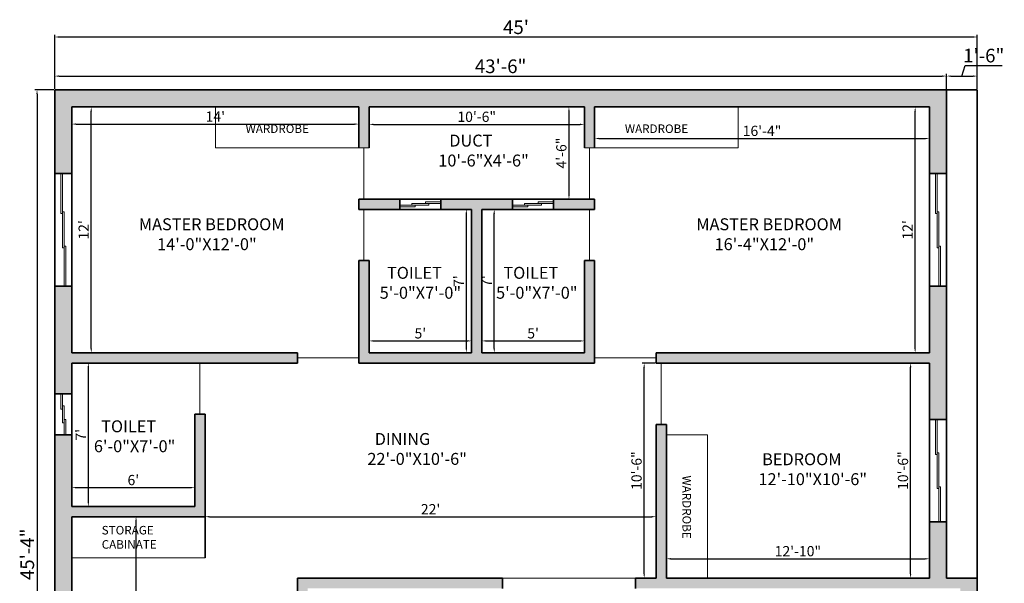
# Model space of a CAD drawing. Units: inches. Extents: x 3491 to 6898, y 1360 to 2019.
# Tile 9 of 9: x 6321 to 6898, y 1683 to 2013. Entities that reach past the tile are written whole.
import ezdxf

# ---------------------------------------------------------------- set-up
doc = ezdxf.new("R2010")
doc.units = ezdxf.units.IN
for name, color, linetype, lineweight in [('A-ANNO-DIMS', 2, 'Continuous', 18), ('A-ANNO-TEXT', 7, 'Continuous', 18), ('A-AREA-IDEN', 7, 'Continuous', 18), ('A-DOOR', 4, 'Continuous', 18), ('A-FLOR-CASE', 8, 'Continuous', 18), ('A-GLAZ', 5, 'Continuous', 18), ('A-WALL', 7, 'Continuous', 35), ('A-WALL-PATT', 8, 'Continuous', 13)]:
    doc.layers.add(name, color=color, linetype=linetype, lineweight=lineweight)
doc.layers.add('A-WALL-OPEN', color=251, linetype='Continuous', lineweight=13, true_color=0x636466)
doc.styles.get("Standard").update_dxf_attribs({"font": 'arial.ttf'})
doc.dimstyles.new('ISO-25', dxfattribs={"dimtxt": 8, "dimasz": 2.5, "dimexe": 1.25, "dimexo": 0.625, "dimtad": 1, "dimdec": 1, "dimlunit": 3, "dimtxsty": 'Standard', "dimcen": 2.5, "dimclrt": 1, "dimadec": 0, "dimazin": 0, "dimtfac": 1, "dimtdec": 1, "dimtmove": 0, "dimatfit": 3, "dimfxl": 1, "dimarcsym": 0})

# ---------------------------------------------------------------- blocks, each defined once
blk = doc.blocks.new('*D33')
at = {"layer": 'A-ANNO-DIMS', "color": 0, "lineweight": -2, "transparency": 16777216}
for p, q in [((6341.78, 1972.99), (6341.78, 1981.69)), ((6344.28, 1980.44), (6861.28, 1980.44)), ((6863.78, 1972.99), (6863.78, 1981.69))]:
    blk.add_line(p, q, dxfattribs=at)
at = {"layer": 'A-ANNO-DIMS', "color": 0, "transparency": 16777216}
for points in [[(6344.28, 1980.85), (6344.28, 1980.02), (6341.78, 1980.44)], [(6861.28, 1980.85), (6861.28, 1980.02), (6863.78, 1980.44)]]:
    blk.add_solid(points, dxfattribs=at)
at = {"layer": 'Defpoints', "color": 0, "transparency": 16777216}
for p in [(6863.78, 1980.44), (6341.78, 1972.37), (6863.78, 1972.37)]:
    blk.add_point(p, dxfattribs=at)
at = {"layer": 'A-ANNO-DIMS', "color": 0, "transparency": 16777216, "insert": (6602.78, 1985.15), "char_height": 8, "attachment_point": 5}
blk.add_mtext('43\'-6"', dxfattribs=at)
blk = doc.blocks.new('*D34')
at = {"layer": 'A-ANNO-DIMS', "color": 0, "lineweight": -2, "transparency": 16777216}
for p, q in [((6872.78, 1980.44), (6874.67, 1986.71)), ((6874.67, 1986.71), (6896.43, 1986.71)), ((6863.78, 1972.99), (6863.78, 1981.69)), ((6866.28, 1980.44), (6879.28, 1980.44)), ((6881.78, 1972.99), (6881.78, 1981.69))]:
    blk.add_line(p, q, dxfattribs=at)
at = {"layer": 'A-ANNO-DIMS', "color": 0, "transparency": 16777216}
for points in [[(6866.28, 1980.85), (6866.28, 1980.02), (6863.78, 1980.44)], [(6879.28, 1980.85), (6879.28, 1980.02), (6881.78, 1980.44)]]:
    blk.add_solid(points, dxfattribs=at)
at = {"layer": 'Defpoints', "color": 0, "transparency": 16777216}
for p in [(6881.78, 1980.44), (6863.78, 1972.37), (6881.78, 1972.37)]:
    blk.add_point(p, dxfattribs=at)
at = {"layer": 'A-ANNO-DIMS', "color": 0, "transparency": 16777216, "insert": (6885.55, 1991.42), "char_height": 8, "attachment_point": 5}
blk.add_mtext('1\'-6"', dxfattribs=at)
blk = doc.blocks.new('*D29')
at = {"layer": 'A-ANNO-DIMS', "color": 0, "lineweight": -2, "transparency": 16777216}
for p, q in [((6341.78, 1972.99), (6341.78, 2004.59)), ((6344.28, 2003.34), (6879.28, 2003.34)), ((6881.78, 1972.99), (6881.78, 2004.59))]:
    blk.add_line(p, q, dxfattribs=at)
at = {"layer": 'A-ANNO-DIMS', "color": 0, "transparency": 16777216}
for points in [[(6344.28, 2003.76), (6344.28, 2002.92), (6341.78, 2003.34)], [(6879.28, 2003.76), (6879.28, 2002.92), (6881.78, 2003.34)]]:
    blk.add_solid(points, dxfattribs=at)
at = {"layer": 'Defpoints', "color": 0, "transparency": 16777216}
for p in [(6881.78, 2003.34), (6341.78, 1972.37), (6881.78, 1972.37)]:
    blk.add_point(p, dxfattribs=at)
at = {"layer": 'A-ANNO-DIMS', "color": 0, "transparency": 16777216, "insert": (6611.78, 2008.03), "char_height": 8, "attachment_point": 5}
blk.add_mtext("45'", dxfattribs=at)
blk = doc.blocks.new('*D35')
at = {"layer": 'A-ANNO-DIMS', "color": 0, "lineweight": -2, "transparency": 16777216}
for p, q in [((6341.16, 1972.37), (6330.15, 1972.37)), ((6331.4, 1969.87), (6331.4, 1430.87)), ((6341.16, 1428.37), (6330.15, 1428.37))]:
    blk.add_line(p, q, dxfattribs=at)
at = {"layer": 'A-ANNO-DIMS', "color": 0, "transparency": 16777216}
for points in [[(6330.99, 1969.87), (6331.82, 1969.87), (6331.4, 1972.37)], [(6330.99, 1430.87), (6331.82, 1430.87), (6331.4, 1428.37)]]:
    blk.add_solid(points, dxfattribs=at)
at = {"layer": 'Defpoints', "color": 0, "transparency": 16777216}
for p in [(6341.78, 1972.37), (6331.4, 1428.37), (6341.78, 1428.37)]:
    blk.add_point(p, dxfattribs=at)
at = {"layer": 'A-ANNO-DIMS', "color": 0, "transparency": 16777216, "insert": (6326.71, 1700.37), "char_height": 8, "attachment_point": 5, "rotation": 90}
blk.add_mtext('45\'-4"', dxfattribs=at)
blk = doc.blocks.new('*D76')
at = {"layer": 'A-ANNO-DIMS', "color": 0, "lineweight": -2, "transparency": 16777216}
for p, q in [((6352.41, 1722.37), (6390.61, 1722.37)), ((6389.36, 1534.87), (6389.36, 1719.87)), ((6352.41, 1532.37), (6390.61, 1532.37))]:
    blk.add_line(p, q, dxfattribs=at)
at = {"layer": 'A-ANNO-DIMS', "color": 0, "transparency": 16777216}
for points in [[(6388.94, 1719.87), (6389.78, 1719.87), (6389.36, 1722.37)], [(6388.94, 1534.87), (6389.78, 1534.87), (6389.36, 1532.37)]]:
    blk.add_solid(points, dxfattribs=at)
at = {"layer": 'Defpoints', "color": 0, "transparency": 16777216}
for p in [(6351.78, 1722.37), (6389.36, 1722.37), (6351.78, 1532.37)]:
    blk.add_point(p, dxfattribs=at)
at = {"layer": 'A-ANNO-DIMS', "color": 0, "transparency": 16777216, "insert": (6385.67, 1627.37), "char_height": 6, "attachment_point": 5, "rotation": 90}
blk.add_mtext('15\'-10"', dxfattribs=at)
blk = doc.blocks.new('*D83')
at = {"layer": 'A-ANNO-DIMS', "color": 0, "lineweight": -2, "transparency": 16777216}
for p, q in [((6699.78, 1686.99), (6699.78, 1698.98)), ((6702.28, 1697.73), (6851.28, 1697.73)), ((6853.78, 1686.99), (6853.78, 1698.98))]:
    blk.add_line(p, q, dxfattribs=at)
at = {"layer": 'A-ANNO-DIMS', "color": 0, "transparency": 16777216}
for points in [[(6702.28, 1698.15), (6702.28, 1697.31), (6699.78, 1697.73)], [(6851.28, 1698.15), (6851.28, 1697.31), (6853.78, 1697.73)]]:
    blk.add_solid(points, dxfattribs=at)
at = {"layer": 'Defpoints', "color": 0, "transparency": 16777216}
for p in [(6853.78, 1697.73), (6699.78, 1686.37), (6853.78, 1686.37)]:
    blk.add_point(p, dxfattribs=at)
at = {"layer": 'A-ANNO-DIMS', "color": 0, "transparency": 16777216, "insert": (6776.78, 1701.42), "char_height": 6, "attachment_point": 5}
blk.add_mtext('12\'-10"', dxfattribs=at)
blk = doc.blocks.new('*D84')
at = {"layer": 'A-ANNO-DIMS', "color": 0, "lineweight": -2, "transparency": 16777216}
for p, q in [((6853.16, 1812.37), (6841.5, 1812.37)), ((6842.75, 1688.87), (6842.75, 1809.87)), ((6853.16, 1686.37), (6841.5, 1686.37))]:
    blk.add_line(p, q, dxfattribs=at)
at = {"layer": 'A-ANNO-DIMS', "color": 0, "transparency": 16777216}
for points in [[(6842.34, 1809.87), (6843.17, 1809.87), (6842.75, 1812.37)], [(6842.34, 1688.87), (6843.17, 1688.87), (6842.75, 1686.37)]]:
    blk.add_solid(points, dxfattribs=at)
at = {"layer": 'Defpoints', "color": 0, "transparency": 16777216}
for p in [(6842.75, 1812.37), (6853.78, 1812.37), (6853.78, 1686.37)]:
    blk.add_point(p, dxfattribs=at)
at = {"layer": 'A-ANNO-DIMS', "color": 0, "transparency": 16777216, "insert": (6839.06, 1749.37), "char_height": 6, "attachment_point": 5, "rotation": 90}
blk.add_mtext('10\'-6"', dxfattribs=at)
blk = doc.blocks.new('*D85')
at = {"layer": 'A-ANNO-DIMS', "color": 0, "lineweight": -2, "transparency": 16777216}
for p, q in [((6853.16, 1962.37), (6844.17, 1962.37)), ((6845.42, 1820.87), (6845.42, 1959.87)), ((6853.16, 1818.37), (6844.17, 1818.37))]:
    blk.add_line(p, q, dxfattribs=at)
at = {"layer": 'A-ANNO-DIMS', "color": 0, "transparency": 16777216}
for points in [[(6845, 1959.87), (6845.84, 1959.87), (6845.42, 1962.37)], [(6845, 1820.87), (6845.84, 1820.87), (6845.42, 1818.37)]]:
    blk.add_solid(points, dxfattribs=at)
at = {"layer": 'Defpoints', "color": 0, "transparency": 16777216}
for p in [(6845.42, 1962.37), (6853.78, 1962.37), (6853.78, 1818.37)]:
    blk.add_point(p, dxfattribs=at)
at = {"layer": 'A-ANNO-DIMS', "color": 0, "transparency": 16777216, "insert": (6841.78, 1890.37), "char_height": 6, "attachment_point": 5, "rotation": 90}
blk.add_mtext("12'", dxfattribs=at)
blk = doc.blocks.new('*D86')
at = {"layer": 'A-ANNO-DIMS', "color": 0, "lineweight": -2, "transparency": 16777216}
for p, q in [((6657.78, 1961.74), (6657.78, 1942.63)), ((6853.78, 1961.74), (6853.78, 1942.63)), ((6660.28, 1943.88), (6851.28, 1943.88))]:
    blk.add_line(p, q, dxfattribs=at)
at = {"layer": 'A-ANNO-DIMS', "color": 0, "transparency": 16777216}
for points in [[(6660.28, 1944.3), (6660.28, 1943.47), (6657.78, 1943.88)], [(6851.28, 1944.3), (6851.28, 1943.47), (6853.78, 1943.88)]]:
    blk.add_solid(points, dxfattribs=at)
at = {"layer": 'Defpoints', "color": 0, "transparency": 16777216}
for p in [(6657.78, 1962.37), (6853.78, 1962.37), (6853.78, 1943.88)]:
    blk.add_point(p, dxfattribs=at)
at = {"layer": 'A-ANNO-DIMS', "color": 0, "transparency": 16777216, "insert": (6755.78, 1947.57), "char_height": 6, "attachment_point": 5}
blk.add_mtext('16\'-4"', dxfattribs=at)
blk = doc.blocks.new('*D87')
at = {"layer": 'A-ANNO-DIMS', "color": 0, "lineweight": -2, "transparency": 16777216}
for p, q in [((6525.78, 1961.74), (6525.78, 1950.9)), ((6651.78, 1961.74), (6651.78, 1950.9)), ((6528.28, 1952.15), (6649.28, 1952.15))]:
    blk.add_line(p, q, dxfattribs=at)
at = {"layer": 'A-ANNO-DIMS', "color": 0, "transparency": 16777216}
for points in [[(6528.28, 1952.57), (6528.28, 1951.74), (6525.78, 1952.15)], [(6649.28, 1952.57), (6649.28, 1951.74), (6651.78, 1952.15)]]:
    blk.add_solid(points, dxfattribs=at)
at = {"layer": 'Defpoints', "color": 0, "transparency": 16777216}
for p in [(6525.78, 1962.37), (6651.78, 1962.37), (6651.78, 1952.15)]:
    blk.add_point(p, dxfattribs=at)
at = {"layer": 'A-ANNO-DIMS', "color": 0, "transparency": 16777216, "insert": (6588.78, 1955.84), "char_height": 6, "attachment_point": 5}
blk.add_mtext('10\'-6"', dxfattribs=at)
blk = doc.blocks.new('*D88')
at = {"layer": 'A-ANNO-DIMS', "color": 0, "lineweight": -2, "transparency": 16777216}
for p, q in [((6351.78, 1961.74), (6351.78, 1951.1)), ((6519.78, 1961.74), (6519.78, 1951.1)), ((6354.28, 1952.35), (6517.28, 1952.35))]:
    blk.add_line(p, q, dxfattribs=at)
at = {"layer": 'A-ANNO-DIMS', "color": 0, "transparency": 16777216}
for points in [[(6354.28, 1952.76), (6354.28, 1951.93), (6351.78, 1952.35)], [(6517.28, 1952.76), (6517.28, 1951.93), (6519.78, 1952.35)]]:
    blk.add_solid(points, dxfattribs=at)
at = {"layer": 'Defpoints', "color": 0, "transparency": 16777216}
for p in [(6351.78, 1962.37), (6519.78, 1962.37), (6519.78, 1952.35)]:
    blk.add_point(p, dxfattribs=at)
at = {"layer": 'A-ANNO-DIMS', "color": 0, "transparency": 16777216, "insert": (6435.78, 1955.98), "char_height": 6, "attachment_point": 5}
blk.add_mtext("14'", dxfattribs=at)
blk = doc.blocks.new('*D89')
at = {"layer": 'A-ANNO-DIMS', "color": 0, "lineweight": -2, "transparency": 16777216}
for p, q in [((6352.41, 1962.37), (6364.38, 1962.37)), ((6363.13, 1820.87), (6363.13, 1959.87)), ((6352.41, 1818.37), (6364.38, 1818.37))]:
    blk.add_line(p, q, dxfattribs=at)
at = {"layer": 'A-ANNO-DIMS', "color": 0, "transparency": 16777216}
for points in [[(6362.71, 1959.87), (6363.55, 1959.87), (6363.13, 1962.37)], [(6362.71, 1820.87), (6363.55, 1820.87), (6363.13, 1818.37)]]:
    blk.add_solid(points, dxfattribs=at)
at = {"layer": 'Defpoints', "color": 0, "transparency": 16777216}
for p in [(6351.78, 1962.37), (6363.13, 1962.37), (6351.78, 1818.37)]:
    blk.add_point(p, dxfattribs=at)
at = {"layer": 'A-ANNO-DIMS', "color": 0, "transparency": 16777216, "insert": (6359.49, 1890.37), "char_height": 6, "attachment_point": 5, "rotation": 90}
blk.add_mtext("12'", dxfattribs=at)
blk = doc.blocks.new('*D90')
at = {"layer": 'A-ANNO-DIMS', "color": 0, "lineweight": -2, "transparency": 16777216}
for p, q in [((6525.78, 1818.99), (6525.78, 1826.58)), ((6528.28, 1825.33), (6583.28, 1825.33)), ((6585.78, 1818.99), (6585.78, 1826.58))]:
    blk.add_line(p, q, dxfattribs=at)
at = {"layer": 'A-ANNO-DIMS', "color": 0, "transparency": 16777216}
for points in [[(6528.28, 1825.75), (6528.28, 1824.92), (6525.78, 1825.33)], [(6583.28, 1825.75), (6583.28, 1824.92), (6585.78, 1825.33)]]:
    blk.add_solid(points, dxfattribs=at)
at = {"layer": 'Defpoints', "color": 0, "transparency": 16777216}
for p in [(6585.78, 1825.33), (6525.78, 1818.37), (6585.78, 1818.37)]:
    blk.add_point(p, dxfattribs=at)
at = {"layer": 'A-ANNO-DIMS', "color": 0, "transparency": 16777216, "insert": (6555.78, 1829.01), "char_height": 6, "attachment_point": 5}
blk.add_mtext("5'", dxfattribs=at)
blk = doc.blocks.new('*D91')
at = {"layer": 'A-ANNO-DIMS', "color": 0, "lineweight": -2, "transparency": 16777216}
for p, q in [((6585.16, 1902.37), (6581.45, 1902.37)), ((6582.7, 1820.87), (6582.7, 1899.87)), ((6585.16, 1818.37), (6581.45, 1818.37))]:
    blk.add_line(p, q, dxfattribs=at)
at = {"layer": 'A-ANNO-DIMS', "color": 0, "transparency": 16777216}
for points in [[(6582.28, 1899.87), (6583.11, 1899.87), (6582.7, 1902.37)], [(6582.28, 1820.87), (6583.11, 1820.87), (6582.7, 1818.37)]]:
    blk.add_solid(points, dxfattribs=at)
at = {"layer": 'Defpoints', "color": 0, "transparency": 16777216}
for p in [(6582.7, 1902.37), (6585.78, 1902.37), (6585.78, 1818.37)]:
    blk.add_point(p, dxfattribs=at)
at = {"layer": 'A-ANNO-DIMS', "color": 0, "transparency": 16777216, "insert": (6579.07, 1860.37), "char_height": 6, "attachment_point": 5, "rotation": 90}
blk.add_mtext("7'", dxfattribs=at)
blk = doc.blocks.new('*D92')
at = {"layer": 'A-ANNO-DIMS', "color": 0, "lineweight": -2, "transparency": 16777216}
for p, q in [((6592.41, 1902.37), (6600.28, 1902.37)), ((6599.03, 1820.87), (6599.03, 1899.87)), ((6592.41, 1818.37), (6600.28, 1818.37))]:
    blk.add_line(p, q, dxfattribs=at)
at = {"layer": 'A-ANNO-DIMS', "color": 0, "transparency": 16777216}
for points in [[(6598.62, 1899.87), (6599.45, 1899.87), (6599.03, 1902.37)], [(6598.62, 1820.87), (6599.45, 1820.87), (6599.03, 1818.37)]]:
    blk.add_solid(points, dxfattribs=at)
at = {"layer": 'Defpoints', "color": 0, "transparency": 16777216}
for p in [(6591.78, 1902.37), (6599.03, 1902.37), (6591.78, 1818.37)]:
    blk.add_point(p, dxfattribs=at)
at = {"layer": 'A-ANNO-DIMS', "color": 0, "transparency": 16777216, "insert": (6595.41, 1860.37), "char_height": 6, "attachment_point": 5, "rotation": 90}
blk.add_mtext("7'", dxfattribs=at)
blk = doc.blocks.new('*D93')
at = {"layer": 'A-ANNO-DIMS', "color": 0, "lineweight": -2, "transparency": 16777216}
for p, q in [((6591.78, 1818.99), (6591.78, 1826.58)), ((6594.28, 1825.33), (6649.28, 1825.33)), ((6651.78, 1818.99), (6651.78, 1826.58))]:
    blk.add_line(p, q, dxfattribs=at)
at = {"layer": 'A-ANNO-DIMS', "color": 0, "transparency": 16777216}
for points in [[(6594.28, 1825.75), (6594.28, 1824.92), (6591.78, 1825.33)], [(6649.28, 1825.75), (6649.28, 1824.92), (6651.78, 1825.33)]]:
    blk.add_solid(points, dxfattribs=at)
at = {"layer": 'Defpoints', "color": 0, "transparency": 16777216}
for p in [(6651.78, 1825.33), (6591.78, 1818.37), (6651.78, 1818.37)]:
    blk.add_point(p, dxfattribs=at)
at = {"layer": 'A-ANNO-DIMS', "color": 0, "transparency": 16777216, "insert": (6621.78, 1829.01), "char_height": 6, "attachment_point": 5}
blk.add_mtext("5'", dxfattribs=at)
blk = doc.blocks.new('*D94')
at = {"layer": 'A-ANNO-DIMS', "color": 0, "lineweight": -2, "transparency": 16777216}
for p, q in [((6642.77, 1959.87), (6642.77, 1910.87)), ((6643.4, 1962.37), (6644.02, 1962.37)), ((6643.4, 1908.37), (6644.02, 1908.37))]:
    blk.add_line(p, q, dxfattribs=at)
at = {"layer": 'A-ANNO-DIMS', "color": 0, "transparency": 16777216}
for points in [[(6642.36, 1959.87), (6643.19, 1959.87), (6642.77, 1962.37)], [(6642.36, 1910.87), (6643.19, 1910.87), (6642.77, 1908.37)]]:
    blk.add_solid(points, dxfattribs=at)
at = {"layer": 'Defpoints', "color": 0, "transparency": 16777216}
for p in [(6642.77, 1962.37), (6642.77, 1908.37), (6642.77, 1908.37)]:
    blk.add_point(p, dxfattribs=at)
at = {"layer": 'A-ANNO-DIMS', "color": 0, "transparency": 16777216, "insert": (6639.09, 1935.37), "char_height": 6, "attachment_point": 5, "rotation": 90}
blk.add_mtext('4\'-6"', dxfattribs=at)
blk = doc.blocks.new('*D95')
at = {"layer": 'A-ANNO-DIMS', "color": 0, "lineweight": -2, "transparency": 16777216}
for p, q in [((6352.41, 1812.37), (6362.69, 1812.37)), ((6361.44, 1730.87), (6361.44, 1809.87)), ((6352.41, 1728.37), (6362.69, 1728.37))]:
    blk.add_line(p, q, dxfattribs=at)
at = {"layer": 'A-ANNO-DIMS', "color": 0, "transparency": 16777216}
for points in [[(6361.02, 1809.87), (6361.85, 1809.87), (6361.44, 1812.37)], [(6361.02, 1730.87), (6361.85, 1730.87), (6361.44, 1728.37)]]:
    blk.add_solid(points, dxfattribs=at)
at = {"layer": 'Defpoints', "color": 0, "transparency": 16777216}
for p in [(6351.78, 1812.37), (6361.44, 1812.37), (6351.78, 1728.37)]:
    blk.add_point(p, dxfattribs=at)
at = {"layer": 'A-ANNO-DIMS', "color": 0, "transparency": 16777216, "insert": (6357.81, 1770.37), "char_height": 6, "attachment_point": 5, "rotation": 90}
blk.add_mtext("7'", dxfattribs=at)
blk = doc.blocks.new('*D96')
at = {"layer": 'A-ANNO-DIMS', "color": 0, "lineweight": -2, "transparency": 16777216}
for p, q in [((6351.78, 1728.99), (6351.78, 1740.65)), ((6423.78, 1728.99), (6423.78, 1740.65)), ((6354.28, 1739.4), (6421.28, 1739.4))]:
    blk.add_line(p, q, dxfattribs=at)
at = {"layer": 'A-ANNO-DIMS', "color": 0, "transparency": 16777216}
for points in [[(6354.28, 1739.81), (6354.28, 1738.98), (6351.78, 1739.4)], [(6421.28, 1739.81), (6421.28, 1738.98), (6423.78, 1739.4)]]:
    blk.add_solid(points, dxfattribs=at)
at = {"layer": 'Defpoints', "color": 0, "transparency": 16777216}
for p in [(6423.78, 1739.4), (6351.78, 1728.37), (6423.78, 1728.37)]:
    blk.add_point(p, dxfattribs=at)
at = {"layer": 'A-ANNO-DIMS', "color": 0, "transparency": 16777216, "insert": (6387.78, 1743.08), "char_height": 6, "attachment_point": 5}
blk.add_mtext("6'", dxfattribs=at)
blk = doc.blocks.new('*D97')
at = {"layer": 'A-ANNO-DIMS', "color": 0, "lineweight": -2, "transparency": 16777216}
for p, q in [((6429.78, 1722.99), (6429.78, 1723.62)), ((6693.78, 1722.99), (6693.78, 1723.62)), ((6432.28, 1722.37), (6691.28, 1722.37))]:
    blk.add_line(p, q, dxfattribs=at)
at = {"layer": 'A-ANNO-DIMS', "color": 0, "transparency": 16777216}
for points in [[(6432.28, 1722.78), (6432.28, 1721.95), (6429.78, 1722.37)], [(6691.28, 1722.78), (6691.28, 1721.95), (6693.78, 1722.37)]]:
    blk.add_solid(points, dxfattribs=at)
at = {"layer": 'Defpoints', "color": 0, "transparency": 16777216}
for p in [(6429.78, 1722.37), (6693.78, 1722.37), (6693.78, 1722.37)]:
    blk.add_point(p, dxfattribs=at)
at = {"layer": 'A-ANNO-DIMS', "color": 0, "transparency": 16777216, "insert": (6561.78, 1726), "char_height": 6, "attachment_point": 5}
blk.add_mtext("22'", dxfattribs=at)
blk = doc.blocks.new('*D98')
at = {"layer": 'A-ANNO-DIMS', "color": 0, "lineweight": -2, "transparency": 16777216}
for p, q in [((6693.16, 1812.37), (6685.56, 1812.37)), ((6686.81, 1688.87), (6686.81, 1809.87)), ((6687.16, 1686.37), (6685.56, 1686.37))]:
    blk.add_line(p, q, dxfattribs=at)
at = {"layer": 'A-ANNO-DIMS', "color": 0, "transparency": 16777216}
for points in [[(6686.39, 1809.87), (6687.23, 1809.87), (6686.81, 1812.37)], [(6686.39, 1688.87), (6687.23, 1688.87), (6686.81, 1686.37)]]:
    blk.add_solid(points, dxfattribs=at)
at = {"layer": 'Defpoints', "color": 0, "transparency": 16777216}
for p in [(6686.81, 1812.37), (6693.78, 1812.37), (6687.78, 1686.37)]:
    blk.add_point(p, dxfattribs=at)
at = {"layer": 'A-ANNO-DIMS', "color": 0, "transparency": 16777216, "insert": (6683.12, 1749.37), "char_height": 6, "attachment_point": 5, "rotation": 90}
blk.add_mtext('10\'-6"', dxfattribs=at)
blk = doc.blocks.new('WIN-SLIDER-24IN')
for p, q in [((0, 1), (17, 1)), ((0, 0), (9, 0)), ((7, 1), (7, 2)), ((7, 2), (24, 2)), ((9, 0), (9, 1)), ((15, 2), (15, 3)), ((15, 3), (24, 3)), ((17, 1), (17, 2))]:
    blk.add_line(p, q)
blk = doc.blocks.new('WIN-SLIDER-66IN')
for p, q in [((0, 42.5), (0, 66)), ((1, 22.5), (1, 66)), ((1, 42.5), (0, 42.5)), ((2, 43.5), (1, 43.5)), ((2, 0), (2, 43.5)), ((3, 23.5), (2, 23.5)), ((3, 0), (3, 23.5)), ((2, 22.5), (1, 22.5))]:
    blk.add_line(p, q)
blk = doc.blocks.new('WIN-SLIDER-60IN')
for p, q in [((0, 39.5), (0, 60)), ((1, 19.5), (1, 60)), ((2, 40.5), (1, 40.5)), ((2, 0), (2, 40.5)), ((1, 39.5), (0, 39.5)), ((2, 19.5), (1, 19.5)), ((3, 20.5), (2, 20.5)), ((3, 0), (3, 20.5))]:
    blk.add_line(p, q)
blk = doc.blocks.new('WARDROBE-84X24')
for q in [(0, 84), (24, 0)]:
    blk.add_line((24, 84), q)

msp = doc.modelspace()

# ---------------------------------------------------------------- hatches: boundary and pattern name
at = {"layer": 'A-WALL-PATT'}
h = msp.add_hatch(color=256, dxfattribs=at)
h.dxf.hatch_style = 1
h.paths.add_polyline_path([(6665.78, 1532.37), (6657.78, 1532.37), (6633.8, 1532.37), (6633.8, 1522.37), (6665.78, 1522.37)])
h.paths.add_polyline_path([(6715.78, 1556.37), (6705.78, 1556.37), (6705.78, 1532.37), (6701.78, 1532.37), (6701.78, 1522.37), (6705.78, 1522.37), (6705.78, 1486.37), (6742.76, 1486.37), (6742.76, 1496.37), (6715.78, 1496.37)], flags=17)
h.paths.add_polyline_path([(6585.8, 1532.37), (6537.78, 1532.37), (6537.78, 1522.37), (6585.8, 1522.37)], flags=17)
h.paths.add_polyline_path([(6829.78, 1496.37), (6802.76, 1496.37), (6802.76, 1486.37), (6829.78, 1486.37)], flags=17)
h.paths.add_polyline_path([(6881.78, 1686.37), (6863.78, 1686.37), (6863.78, 1719.37), (6853.78, 1719.37), (6853.78, 1686.37), (6699.78, 1686.37), (6699.78, 1776.37), (6693.78, 1776.37), (6693.78, 1686.37), (6681.78, 1686.37), (6681.78, 1680.37), (6871.78, 1680.37), (6871.78, 1496.37), (6859.78, 1496.37), (6859.78, 1486.37), (6881.78, 1486.37)])
h.paths.add_polyline_path([(6603.78, 1686.37), (6483.78, 1686.37), (6483.78, 1532.37), (6465.81, 1532.37), (6465.81, 1522.37), (6495.78, 1522.37), (6495.78, 1532.37), (6489.78, 1532.37), (6489.78, 1680.37), (6603.78, 1680.37)])
h.paths.add_polyline_path([(6351.78, 1722.37), (6429.78, 1722.37), (6429.78, 1782.37), (6423.78, 1782.37), (6423.78, 1728.37), (6351.78, 1728.37), (6351.78, 1770.37), (6341.78, 1770.37), (6341.78, 1628.4), (6351.78, 1628.4)])
h.paths.add_polyline_path([(6351.78, 1580.4), (6341.78, 1580.4), (6341.78, 1428.37), (6483.78, 1428.37), (6483.78, 1438.37), (6351.78, 1438.37), (6351.78, 1522.37), (6417.81, 1522.37), (6417.81, 1532.37), (6351.78, 1532.37)])
h.paths.add_polyline_path([(6549.78, 1486.37), (6543.78, 1486.37), (6543.78, 1428.37), (6549.78, 1428.37)])
h.paths.add_polyline_path([(6863.78, 1857.37), (6853.78, 1857.37), (6853.78, 1818.37), (6693.78, 1818.37), (6693.78, 1812.37), (6853.78, 1812.37), (6853.78, 1779.37), (6863.78, 1779.37)])
h.paths.add_polyline_path([(6657.78, 1872.37), (6651.78, 1872.37), (6651.78, 1818.37), (6591.78, 1818.37), (6591.78, 1902.37), (6609.78, 1902.37), (6609.78, 1908.37), (6567.78, 1908.37), (6567.78, 1902.37), (6585.78, 1902.37), (6585.78, 1818.37), (6525.78, 1818.37), (6525.78, 1872.37), (6519.78, 1872.37), (6519.78, 1812.37), (6657.78, 1812.37)])
h.paths.add_polyline_path([(6351.78, 1857.37), (6341.78, 1857.37), (6341.78, 1794.37), (6351.78, 1794.37), (6351.78, 1812.37), (6483.78, 1812.37), (6483.78, 1818.37), (6351.78, 1818.37)])
h.paths.add_polyline_path([(6351.78, 1962.37), (6519.78, 1962.37), (6519.78, 1938.37), (6525.78, 1938.37), (6525.78, 1962.37), (6651.78, 1962.37), (6651.78, 1938.37), (6657.78, 1938.37), (6657.78, 1962.37), (6853.78, 1962.37), (6853.78, 1923.37), (6863.78, 1923.37), (6863.78, 1972.37), (6341.78, 1972.37), (6341.78, 1923.37), (6351.78, 1923.37)])
h.paths.add_polyline_path([(6657.78, 1908.37), (6633.78, 1908.37), (6633.78, 1902.37), (6657.78, 1902.37)], flags=17)
h.paths.add_polyline_path([(6543.78, 1908.37), (6519.78, 1908.37), (6519.78, 1902.37), (6543.78, 1902.37)], flags=17)

# ---------------------------------------------------------------- linework, layer by layer
at = {"layer": 'A-DOOR'}
for p, q in [((6522.78, 1938.37), (6522.78, 1908.37)), ((6654.78, 1938.37), (6654.78, 1908.37)), ((6522.78, 1872.37), (6522.78, 1902.37)), ((6654.78, 1872.37), (6654.78, 1902.37)), ((6426.78, 1782.37), (6426.78, 1812.37)), ((6483.78, 1815.37), (6519.78, 1815.37)), ((6693.78, 1815.37), (6657.78, 1815.37)), ((6696.78, 1776.37), (6696.78, 1812.37))]:
    msp.add_line(p, q, dxfattribs=at)
at = {"layer": 'A-FLOR-CASE'}
for p, q in [((6435.78, 1962.37), (6435.78, 1938.37)), ((6741.78, 1962.37), (6741.78, 1938.37)), ((6525.78, 1938.37), (6435.78, 1938.37)), ((6741.78, 1938.37), (6651.78, 1938.37)), ((6429.78, 1698.37), (6351.78, 1698.37))]:
    msp.add_line(p, q, dxfattribs=at)
at = {"layer": 'A-WALL'}
for p, q in [((6881.78, 1972.37), (6341.78, 1972.37)), ((6341.78, 1972.37), (6341.78, 1428.37)), ((6863.78, 1972.37), (6863.78, 1686.37)), ((6881.78, 1428.37), (6881.78, 1972.37)), ((6519.78, 1962.37), (6351.78, 1962.37)), ((6351.78, 1962.37), (6351.78, 1818.37)), ((6519.78, 1962.37), (6519.78, 1938.37)), ((6651.78, 1962.37), (6525.78, 1962.37)), ((6525.78, 1962.37), (6525.78, 1938.37)), ((6651.78, 1962.37), (6651.78, 1938.37)), ((6853.78, 1962.37), (6657.78, 1962.37)), ((6657.78, 1962.37), (6657.78, 1938.37)), ((6853.78, 1962.37), (6853.78, 1818.37)), ((6351.78, 1923.37), (6341.78, 1923.37)), ((6863.78, 1923.37), (6853.78, 1923.37)), ((6519.78, 1908.37), (6519.78, 1902.37)), ((6657.78, 1908.37), (6519.78, 1908.37)), ((6543.78, 1908.37), (6543.78, 1902.37)), ((6567.78, 1908.37), (6567.78, 1902.37)), ((6609.78, 1908.37), (6609.78, 1902.37)), ((6633.78, 1908.37), (6633.78, 1902.37)), ((6657.78, 1908.37), (6657.78, 1902.37)), ((6585.78, 1902.37), (6519.78, 1902.37)), ((6585.78, 1902.37), (6585.78, 1818.37)), ((6591.78, 1902.37), (6591.78, 1818.37)), ((6657.78, 1902.37), (6591.78, 1902.37)), ((6519.78, 1872.37), (6519.78, 1812.37)), ((6525.78, 1872.37), (6519.78, 1872.37)), ((6525.78, 1872.37), (6525.78, 1818.37)), ((6651.78, 1872.37), (6651.78, 1818.37)), ((6657.78, 1872.37), (6651.78, 1872.37)), ((6657.78, 1872.37), (6657.78, 1812.37)), ((6351.78, 1857.37), (6341.78, 1857.37)), ((6863.78, 1857.37), (6853.78, 1857.37)), ((6483.78, 1818.37), (6351.78, 1818.37)), ((6483.78, 1818.37), (6483.78, 1812.37)), ((6585.78, 1818.37), (6525.78, 1818.37)), ((6651.78, 1818.37), (6591.78, 1818.37)), ((6853.78, 1818.37), (6693.78, 1818.37)), ((6693.78, 1818.37), (6693.78, 1812.37)), ((6483.78, 1812.37), (6351.78, 1812.37)), ((6351.78, 1812.37), (6351.78, 1728.37)), ((6657.78, 1812.37), (6519.78, 1812.37)), ((6853.78, 1812.37), (6693.78, 1812.37)), ((6853.78, 1812.37), (6853.78, 1686.37)), ((6351.78, 1794.37), (6341.78, 1794.37)), ((6429.78, 1782.37), (6423.78, 1782.37)), ((6423.78, 1782.37), (6423.78, 1728.37)), ((6429.78, 1782.37), (6429.78, 1698.37)), ((6699.78, 1776.37), (6693.78, 1776.37)), ((6693.78, 1776.37), (6693.78, 1686.37)), ((6699.78, 1776.37), (6699.78, 1686.37)), ((6863.78, 1779.37), (6853.78, 1779.37)), ((6351.78, 1770.37), (6341.78, 1770.37)), ((6423.78, 1728.37), (6351.78, 1728.37)), ((6429.78, 1722.37), (6351.78, 1722.37)), ((6351.78, 1722.37), (6351.78, 1532.37)), ((6863.78, 1719.37), (6853.78, 1719.37)), ((6603.78, 1686.37), (6483.78, 1686.37)), ((6483.78, 1686.37), (6483.78, 1532.37)), ((6603.78, 1686.37), (6603.78, 1680.37)), ((6693.78, 1686.37), (6681.78, 1686.37)), ((6681.78, 1686.37), (6681.78, 1680.37)), ((6853.78, 1686.37), (6699.78, 1686.37)), ((6881.78, 1686.37), (6863.78, 1686.37))]:
    msp.add_line(p, q, dxfattribs=at)
at = {"layer": 'A-WALL-OPEN'}
msp.add_line((6681.78, 1686.37), (6603.78, 1686.37), dxfattribs=at)

# ---------------------------------------------------------------- block references
at = {"layer": 'A-FLOR-CASE'}
msp.add_blockref('WARDROBE-84X24', (6699.78, 1686.37), dxfattribs=at)
at = {"layer": 'A-GLAZ'}
for name, p in [('WIN-SLIDER-66IN', (6345.28, 1857.37)), ('WIN-SLIDER-66IN', (6857.28, 1857.37)), ('WIN-SLIDER-24IN', (6543.78, 1903.87)), ('WIN-SLIDER-24IN', (6609.78, 1903.87)), ('WIN-SLIDER-60IN', (6857.28, 1719.37))]:
    msp.add_blockref(name, p, dxfattribs=at)
at = {"layer": 'A-GLAZ', "rotation": 270}
msp.add_blockref('WIN-SLIDER-24IN', (6345.28, 1794.37), dxfattribs=at)

# ---------------------------------------------------------------- texts
at = {"layer": 'A-ANNO-TEXT', "char_height": 5, "attachment_point": 1}
for s, insert in [('WARDROBE', (6453.49, 1952.13)), ('WARDROBE', (6675.49, 1952.13)), ('STORAGE\\PCABINATE', (6369.27, 1716.98))]:
    msp.add_mtext_dynamic_manual_height_columns(s, width=86.9528, gutter_width=12.5, heights=[0], dxfattribs=dict(at, insert=insert))
at = {"layer": 'A-ANNO-TEXT', "insert": (6714.23, 1746.53), "char_height": 5, "attachment_point": 1, "rotation": 270}
msp.add_mtext_dynamic_manual_height_columns('WARDROBE', width=86.9528, gutter_width=12.5, heights=[0], dxfattribs=at)
at = {"layer": 'A-AREA-IDEN', "char_height": 7, "attachment_point": 1}
for s, heights, insert in [('   DUCT\\P10\'-6"X4\'-6"', [0], (6566.29, 1946.16)), ('MASTER BEDROOM\\P     14\'-0"X12\'-0"', [0], (6391.02, 1897.15)), ('MASTER BEDROOM\\P     16\'-4"X12\'-0"', [0], (6717.31, 1897.15)), ('  TOILET\\P5\'-0"X7\'-0"', [0], (6531.98, 1868.72)), ('  TOILET\\P5\'-0"X7\'-0"', [0], (6600.12, 1868.72)), ('  TOILET\\P6\'-0"X7\'-0"', [0], (6364.7, 1778.82)), ('  DINING\\P22\'-0"X10\'-6"', [18.93], (6524.79, 1771.4)), (' BEDROOM\\P12\'-10"X10\'-6"', [0], (6753.7, 1759.53))]:
    msp.add_mtext_dynamic_manual_height_columns(s, width=121.6144, gutter_width=12.5, heights=heights, dxfattribs=dict(at, insert=insert))

# ---------------------------------------------------------------- dimensions: what is measured, and where the dimension line sits
at = {"layer": 'A-ANNO-DIMS'}
for base, p1, p2, override, picture, middle in [((6881.78, 2003.34), (6341.78, 1972.37), (6881.78, 1972.37), {"dimclrd": 0, "dimclre": 0, "dimclrt": 0}, '*D29', (6611.78, 2008.03)), ((6881.78, 1980.44), (6863.78, 1972.37), (6881.78, 1972.37), {"dimclrd": 0, "dimclre": 0, "dimclrt": 0, "dimtmove": 1}, '*D34', (6875.29, 1991.42)), ((6863.78, 1980.44), (6341.78, 1972.37), (6863.78, 1972.37), {"dimclrd": 0, "dimclre": 0, "dimclrt": 0}, '*D33', (6602.78, 1985.15)), ((6519.78, 1952.35), (6351.78, 1962.37), (6519.78, 1962.37), {"dimtxt": 6, "dimclrd": 0, "dimclre": 0, "dimclrt": 0}, '*D88', (6435.78, 1955.98)), ((6651.78, 1952.15), (6525.78, 1962.37), (6651.78, 1962.37), {"dimtxt": 6, "dimclrd": 0, "dimclre": 0, "dimclrt": 0}, '*D87', (6588.78, 1955.84)), ((6853.78, 1943.88), (6657.78, 1962.37), (6853.78, 1962.37), {"dimtxt": 6, "dimclrd": 0, "dimclre": 0, "dimclrt": 0}, '*D86', (6755.78, 1947.57)), ((6585.78, 1825.33), (6525.78, 1818.37), (6585.78, 1818.37), {"dimtxt": 6, "dimclrd": 0, "dimclre": 0, "dimclrt": 0}, '*D90', (6555.78, 1829.01)), ((6651.78, 1825.33), (6591.78, 1818.37), (6651.78, 1818.37), {"dimtxt": 6, "dimclrd": 0, "dimclre": 0, "dimclrt": 0}, '*D93', (6621.78, 1829.01)), ((6423.78, 1739.4), (6351.78, 1728.37), (6423.78, 1728.37), {"dimtxt": 6, "dimclrd": 0, "dimclre": 0, "dimclrt": 0}, '*D96', (6387.78, 1743.08)), ((6693.78, 1722.37), (6429.78, 1722.37), (6693.78, 1722.37), {"dimtxt": 6, "dimclrd": 0, "dimclre": 0, "dimclrt": 0}, '*D97', (6561.78, 1726)), ((6853.78, 1697.73), (6699.78, 1686.37), (6853.78, 1686.37), {"dimtxt": 6, "dimclrd": 0, "dimclre": 0, "dimclrt": 0}, '*D83', (6776.78, 1701.42))]:
    dim = msp.add_linear_dim(base=base, p1=p1, p2=p2, dimstyle='ISO-25', override=override, dxfattribs=at)
    dim.commit()
    dim.dimension.update_dxf_attribs({"geometry": picture, "text_midpoint": middle})
for base, p1, p2, angle, override, picture, middle in [((6331.4, 1428.37), (6341.78, 1972.37), (6341.78, 1428.37), 90, {"dimclrd": 0, "dimclre": 0, "dimclrt": 0}, '*D35', (6326.71, 1700.37)), ((6363.13, 1962.37), (6351.78, 1818.37), (6351.78, 1962.37), 270, {"dimtxt": 6, "dimclrd": 0, "dimclre": 0, "dimclrt": 0}, '*D89', (6359.49, 1890.37)), ((6642.77, 1908.37), (6642.77, 1962.37), (6642.77, 1908.37), 90, {"dimtxt": 6, "dimclrd": 0, "dimclre": 0, "dimclrt": 0}, '*D94', (6639.09, 1935.37)), ((6845.42, 1962.37), (6853.78, 1818.37), (6853.78, 1962.37), 270, {"dimtxt": 6, "dimclrd": 0, "dimclre": 0, "dimclrt": 0}, '*D85', (6841.78, 1890.37)), ((6582.7, 1902.37), (6585.78, 1818.37), (6585.78, 1902.37), 270, {"dimtxt": 6, "dimclrd": 0, "dimclre": 0, "dimclrt": 0}, '*D91', (6579.07, 1860.37)), ((6599.03, 1902.37), (6591.78, 1818.37), (6591.78, 1902.37), 270, {"dimtxt": 6, "dimclrd": 0, "dimclre": 0, "dimclrt": 0}, '*D92', (6595.41, 1860.37)), ((6361.44, 1812.37), (6351.78, 1728.37), (6351.78, 1812.37), 270, {"dimtxt": 6, "dimclrd": 0, "dimclre": 0, "dimclrt": 0}, '*D95', (6357.81, 1770.37)), ((6686.81, 1812.37), (6687.78, 1686.37), (6693.78, 1812.37), 90, {"dimtxt": 6, "dimclrd": 0, "dimclre": 0, "dimclrt": 0}, '*D98', (6683.12, 1749.37)), ((6842.75, 1812.37), (6853.78, 1686.37), (6853.78, 1812.37), 270, {"dimtxt": 6, "dimclrd": 0, "dimclre": 0, "dimclrt": 0}, '*D84', (6839.06, 1749.37)), ((6389.36, 1722.37), (6351.78, 1532.37), (6351.78, 1722.37), 270, {"dimtxt": 6, "dimclrd": 0, "dimclre": 0, "dimclrt": 0}, '*D76', (6385.67, 1627.37))]:
    dim = msp.add_linear_dim(base=base, p1=p1, p2=p2, angle=angle, dimstyle='ISO-25', override=override, dxfattribs=at)
    dim.commit()
    dim.dimension.update_dxf_attribs({"geometry": picture, "text_midpoint": middle})

doc.saveas('drawing.dxf')
